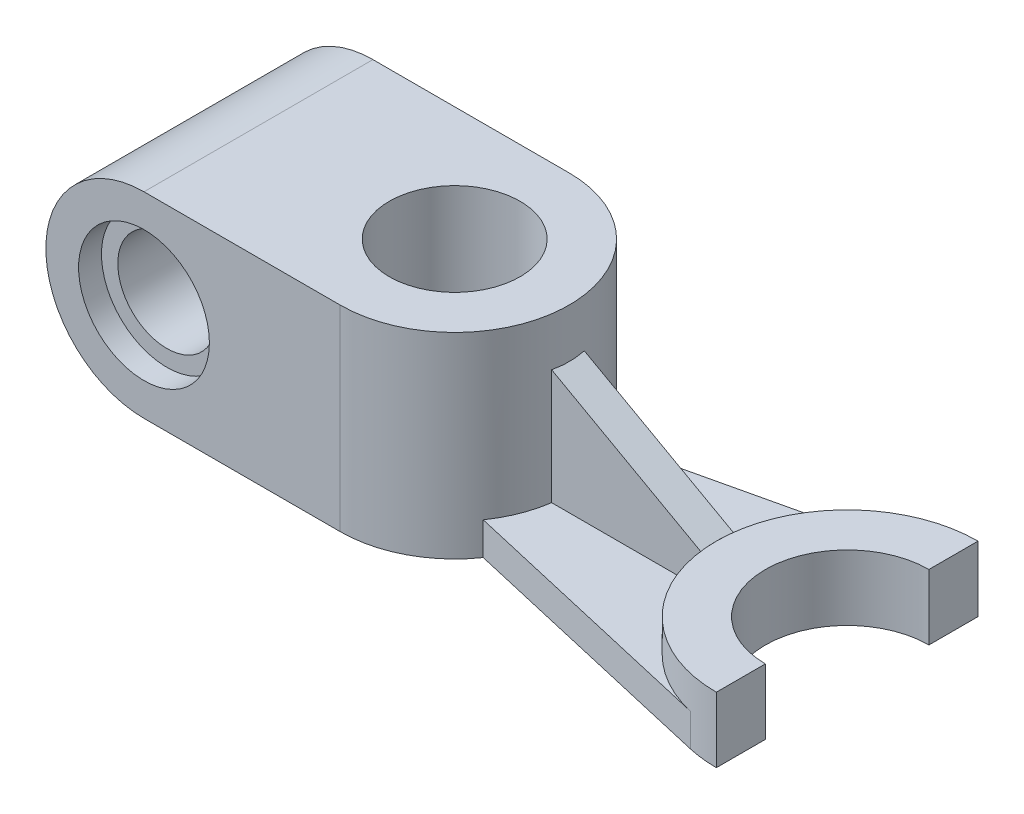
ISO-10303-21;
HEADER;
FILE_DESCRIPTION(('STEP AP214'),'2;1');
FILE_NAME('part.step','',(''),(''),'','','');
FILE_SCHEMA(('AUTOMOTIVE_DESIGN { 1 0 10303 214 1 1 1 1 }'));
ENDSEC;
DATA;
#1=APPLICATION_CONTEXT('core data for automotive mechanical design processes');
#2=APPLICATION_PROTOCOL_DEFINITION('international standard','automotive_design',2000,#1);
#3=PRODUCT_CONTEXT('',#1,'mechanical');
#4=PRODUCT('Part','Part','',(#3));
#5=PRODUCT_RELATED_PRODUCT_CATEGORY('part','',(#4));
#6=PRODUCT_DEFINITION_FORMATION('','',#4);
#7=PRODUCT_DEFINITION_CONTEXT('part definition',#1,'design');
#8=PRODUCT_DEFINITION('design','',#6,#7);
#9=PRODUCT_DEFINITION_SHAPE('','',#8);
#10=(LENGTH_UNIT() NAMED_UNIT(*) SI_UNIT(.MILLI.,.METRE.));
#11=(NAMED_UNIT(*) PLANE_ANGLE_UNIT() SI_UNIT($,.RADIAN.));
#12=(NAMED_UNIT(*) SI_UNIT($,.STERADIAN.) SOLID_ANGLE_UNIT());
#13=UNCERTAINTY_MEASURE_WITH_UNIT(LENGTH_MEASURE(1.E-05),#10,'distance_accuracy_value','');
#14=(GEOMETRIC_REPRESENTATION_CONTEXT(3) GLOBAL_UNCERTAINTY_ASSIGNED_CONTEXT((#13)) GLOBAL_UNIT_ASSIGNED_CONTEXT((#10,
#11,#12)) REPRESENTATION_CONTEXT('',''));
#15=CARTESIAN_POINT('',(0.,0.,0.));
#16=DIRECTION('',(0.,0.,1.));
#17=DIRECTION('',(1.,0.,0.));
#18=AXIS2_PLACEMENT_3D('',#15,#16,#17);
#19=CARTESIAN_POINT('',(0.,10.,0.));
#20=DIRECTION('',(0.,1.,0.));
#21=DIRECTION('',(0.,0.,1.));
#22=AXIS2_PLACEMENT_3D('',#19,#20,#21);
#23=PLANE('',#22);
#24=CARTESIAN_POINT('',(0.,10.,0.));
#25=DIRECTION('',(0.,-1.,0.));
#26=DIRECTION('',(0.,0.,1.));
#27=AXIS2_PLACEMENT_3D('',#24,#25,#26);
#28=CIRCLE('',#27,35.);
#29=CARTESIAN_POINT('',(28.7228132326901,10.,-20.));
#30=VERTEX_POINT('',#29);
#31=CARTESIAN_POINT('',(34.6410161513775,10.,-5.));
#32=VERTEX_POINT('',#31);
#33=EDGE_CURVE('E166',#30,#32,#28,.T.);
#34=ORIENTED_EDGE('',*,*,#33,.T.);
#35=DIRECTION('',(1.,0.,0.));
#36=VECTOR('',#35,1.);
#37=CARTESIAN_POINT('',(0.,10.,-5.));
#38=LINE('',#37,#36);
#39=CARTESIAN_POINT('',(80.3137303340311,10.,-5.));
#40=VERTEX_POINT('',#39);
#41=EDGE_CURVE('E170',#32,#40,#38,.T.);
#42=ORIENTED_EDGE('',*,*,#41,.T.);
#43=CARTESIAN_POINT('',(120.,10.,0.));
#44=DIRECTION('',(0.,-1.,0.));
#45=DIRECTION('',(0.,0.,1.));
#46=AXIS2_PLACEMENT_3D('',#43,#44,#45);
#47=CIRCLE('',#46,40.);
#48=CARTESIAN_POINT('',(111.011327844652,10.,-38.9769646443084));
#49=VERTEX_POINT('',#48);
#50=EDGE_CURVE('E155',#40,#49,#47,.T.);
#51=ORIENTED_EDGE('',*,*,#50,.T.);
#52=DIRECTION('',(-0.97442411610771,0.,0.224716803883704));
#53=VECTOR('',#52,1.);
#54=CARTESIAN_POINT('',(111.011327844652,10.,-38.9769646443084));
#55=LINE('',#54,#53);
#56=EDGE_CURVE('E245',#49,#30,#55,.T.);
#57=ORIENTED_EDGE('',*,*,#56,.T.);
#58=EDGE_LOOP('',(#34,#42,#51,#57));
#59=FACE_BOUND('',#58,.T.);
#60=ADVANCED_FACE('F39',(#59),#23,.T.);
#61=CARTESIAN_POINT('',(120.,20.,0.));
#62=DIRECTION('',(0.,-1.,0.));
#63=DIRECTION('',(0.,0.,-1.));
#64=AXIS2_PLACEMENT_3D('',#61,#62,#63);
#65=CYLINDRICAL_SURFACE('',#64,40.);
#66=CARTESIAN_POINT('',(120.,-2.22222222222223,0.));
#67=DIRECTION('',(-0.485642931178632,-0.874157276121538,0.));
#68=DIRECTION('',(0.874157276121538,-0.485642931178632,0.));
#69=AXIS2_PLACEMENT_3D('',#66,#67,#68);
#70=ELLIPSE('',#69,45.7583561821644,40.);
#71=CARTESIAN_POINT('',(80.,20.,0.));
#72=VERTEX_POINT('',#71);
#73=CARTESIAN_POINT('',(80.3137303340311,19.8257053699827,5.));
#74=VERTEX_POINT('',#73);
#75=EDGE_CURVE('E295',#72,#74,#70,.F.);
#76=ORIENTED_EDGE('',*,*,#75,.T.);
#77=DIRECTION('',(0.,-1.,0.));
#78=VECTOR('',#77,1.);
#79=CARTESIAN_POINT('',(80.3137303340311,20.,5.));
#80=LINE('',#79,#78);
#81=CARTESIAN_POINT('',(80.3137303340311,10.,5.));
#82=VERTEX_POINT('',#81);
#83=EDGE_CURVE('E11',#74,#82,#80,.T.);
#84=ORIENTED_EDGE('',*,*,#83,.T.);
#85=CARTESIAN_POINT('',(111.011327844652,10.,38.9769646443084));
#86=VERTEX_POINT('',#85);
#87=EDGE_CURVE('E162',#86,#82,#47,.T.);
#88=ORIENTED_EDGE('',*,*,#87,.F.);
#89=DIRECTION('',(0.,-1.,0.));
#90=VECTOR('',#89,1.);
#91=CARTESIAN_POINT('',(111.011327844652,10.,38.9769646443084));
#92=LINE('',#91,#90);
#93=CARTESIAN_POINT('',(111.011327844652,0.,38.9769646443084));
#94=VERTEX_POINT('',#93);
#95=EDGE_CURVE('E236',#86,#94,#92,.T.);
#96=ORIENTED_EDGE('',*,*,#95,.T.);
#97=CARTESIAN_POINT('',(120.,0.,0.));
#98=DIRECTION('',(0.,1.,0.));
#99=DIRECTION('',(0.,0.,1.));
#100=AXIS2_PLACEMENT_3D('',#97,#98,#99);
#101=CIRCLE('',#100,40.);
#102=CARTESIAN_POINT('',(120.,0.,40.));
#103=VERTEX_POINT('',#102);
#104=EDGE_CURVE('E271',#94,#103,#101,.T.);
#105=ORIENTED_EDGE('',*,*,#104,.T.);
#106=DIRECTION('',(0.,-1.,0.));
#107=VECTOR('',#106,1.);
#108=CARTESIAN_POINT('',(120.,20.,40.));
#109=LINE('',#108,#107);
#110=CARTESIAN_POINT('',(120.,20.,40.));
#111=VERTEX_POINT('',#110);
#112=EDGE_CURVE('E261',#111,#103,#109,.T.);
#113=ORIENTED_EDGE('',*,*,#112,.F.);
#114=CARTESIAN_POINT('',(120.,20.,0.));
#115=DIRECTION('',(0.,1.,0.));
#116=DIRECTION('',(0.,0.,1.));
#117=AXIS2_PLACEMENT_3D('',#114,#115,#116);
#118=CIRCLE('',#117,40.);
#119=EDGE_CURVE('E285',#72,#111,#118,.T.);
#120=ORIENTED_EDGE('',*,*,#119,.F.);
#121=EDGE_LOOP('',(#76,#84,#88,#96,#105,#113,#120));
#122=FACE_BOUND('',#121,.T.);
#123=ADVANCED_FACE('F310',(#122),#65,.T.);
#124=CARTESIAN_POINT('',(0.,60.,0.));
#125=DIRECTION('',(0.,-1.,0.));
#126=DIRECTION('',(0.,0.,-1.));
#127=AXIS2_PLACEMENT_3D('',#124,#125,#126);
#128=CYLINDRICAL_SURFACE('',#127,35.);
#129=CARTESIAN_POINT('',(34.6410161513775,10.,5.));
#130=VERTEX_POINT('',#129);
#131=CARTESIAN_POINT('',(28.7228132326901,10.,20.));
#132=VERTEX_POINT('',#131);
#133=EDGE_CURVE('E246',#130,#132,#28,.T.);
#134=ORIENTED_EDGE('',*,*,#133,.F.);
#135=DIRECTION('',(0.,-1.,0.));
#136=VECTOR('',#135,1.);
#137=CARTESIAN_POINT('',(34.6410161513775,60.,5.));
#138=LINE('',#137,#136);
#139=CARTESIAN_POINT('',(34.6410161513775,45.1994354714569,5.));
#140=VERTEX_POINT('',#139);
#141=EDGE_CURVE('E53',#130,#140,#138,.F.);
#142=ORIENTED_EDGE('',*,*,#141,.T.);
#143=CARTESIAN_POINT('',(0.,64.4444444444444,0.));
#144=DIRECTION('',(-0.485642931178632,-0.874157276121538,0.));
#145=DIRECTION('',(0.874157276121538,-0.485642931178632,0.));
#146=AXIS2_PLACEMENT_3D('',#143,#144,#145);
#147=ELLIPSE('',#146,40.0385616593939,35.);
#148=CARTESIAN_POINT('',(34.6410161513775,45.1994354714569,-5.));
#149=VERTEX_POINT('',#148);
#150=EDGE_CURVE('E59',#140,#149,#147,.F.);
#151=ORIENTED_EDGE('',*,*,#150,.T.);
#152=DIRECTION('',(0.,-1.,0.));
#153=VECTOR('',#152,1.);
#154=CARTESIAN_POINT('',(34.6410161513775,60.,-5.));
#155=LINE('',#154,#153);
#156=EDGE_CURVE('E167',#32,#149,#155,.F.);
#157=ORIENTED_EDGE('',*,*,#156,.F.);
#158=ORIENTED_EDGE('',*,*,#33,.F.);
#159=DIRECTION('',(0.,-1.,0.));
#160=VECTOR('',#159,1.);
#161=CARTESIAN_POINT('',(28.7228132326901,10.,-20.));
#162=LINE('',#161,#160);
#163=CARTESIAN_POINT('',(28.7228132326901,0.,-20.));
#164=VERTEX_POINT('',#163);
#165=EDGE_CURVE('E237',#30,#164,#162,.T.);
#166=ORIENTED_EDGE('',*,*,#165,.T.);
#167=CARTESIAN_POINT('',(0.,0.,0.));
#168=DIRECTION('',(0.,1.,0.));
#169=DIRECTION('',(0.,0.,1.));
#170=AXIS2_PLACEMENT_3D('',#167,#168,#169);
#171=CIRCLE('',#170,35.);
#172=CARTESIAN_POINT('',(0.,0.,-35.));
#173=VERTEX_POINT('',#172);
#174=EDGE_CURVE('E205',#164,#173,#171,.T.);
#175=ORIENTED_EDGE('',*,*,#174,.T.);
#176=DIRECTION('',(0.,-1.,0.));
#177=VECTOR('',#176,1.);
#178=CARTESIAN_POINT('',(0.,60.,-35.));
#179=LINE('',#178,#177);
#180=CARTESIAN_POINT('',(0.,60.,-35.));
#181=VERTEX_POINT('',#180);
#182=EDGE_CURVE('E176',#181,#173,#179,.T.);
#183=ORIENTED_EDGE('',*,*,#182,.F.);
#184=CARTESIAN_POINT('',(0.,60.,0.));
#185=DIRECTION('',(0.,1.,0.));
#186=DIRECTION('',(0.,0.,1.));
#187=AXIS2_PLACEMENT_3D('',#184,#185,#186);
#188=CIRCLE('',#187,35.);
#189=CARTESIAN_POINT('',(0.,60.,35.));
#190=VERTEX_POINT('',#189);
#191=EDGE_CURVE('E196',#190,#181,#188,.T.);
#192=ORIENTED_EDGE('',*,*,#191,.F.);
#193=DIRECTION('',(0.,-1.,0.));
#194=VECTOR('',#193,1.);
#195=CARTESIAN_POINT('',(0.,60.,35.));
#196=LINE('',#195,#194);
#197=CARTESIAN_POINT('',(0.,0.,35.));
#198=VERTEX_POINT('',#197);
#199=EDGE_CURVE('E178',#190,#198,#196,.T.);
#200=ORIENTED_EDGE('',*,*,#199,.T.);
#201=CARTESIAN_POINT('',(28.7228132326901,0.,20.));
#202=VERTEX_POINT('',#201);
#203=EDGE_CURVE('E199',#198,#202,#171,.T.);
#204=ORIENTED_EDGE('',*,*,#203,.T.);
#205=DIRECTION('',(0.,-1.,0.));
#206=VECTOR('',#205,1.);
#207=CARTESIAN_POINT('',(28.7228132326901,10.,20.));
#208=LINE('',#207,#206);
#209=EDGE_CURVE('E233',#132,#202,#208,.T.);
#210=ORIENTED_EDGE('',*,*,#209,.F.);
#211=EDGE_LOOP('',(#134,#142,#151,#157,#158,#166,#175,#183,#192,#200,#204,#210));
#212=FACE_BOUND('',#211,.T.);
#213=ADVANCED_FACE('F41',(#212),#128,.T.);
#214=CARTESIAN_POINT('',(-60.,30.,-35.));
#215=DIRECTION('',(0.,0.,1.));
#216=DIRECTION('',(1.,0.,0.));
#217=AXIS2_PLACEMENT_3D('',#214,#215,#216);
#218=CYLINDRICAL_SURFACE('',#217,15.);
#219=CARTESIAN_POINT('',(-60.,30.,28.));
#220=DIRECTION('',(0.,0.,1.));
#221=DIRECTION('',(1.,0.,0.));
#222=AXIS2_PLACEMENT_3D('',#219,#220,#221);
#223=CIRCLE('',#222,15.);
#224=CARTESIAN_POINT('',(-45.,30.,28.));
#225=VERTEX_POINT('',#224);
#226=EDGE_CURVE('E187',#225,#225,#223,.F.);
#227=ORIENTED_EDGE('',*,*,#226,.F.);
#228=EDGE_LOOP('',(#227));
#229=FACE_BOUND('',#228,.T.);
#230=CARTESIAN_POINT('',(-60.,30.,-28.));
#231=DIRECTION('',(0.,0.,-1.));
#232=DIRECTION('',(-1.,0.,0.));
#233=AXIS2_PLACEMENT_3D('',#230,#231,#232);
#234=CIRCLE('',#233,15.);
#235=CARTESIAN_POINT('',(-75.,30.,-28.));
#236=VERTEX_POINT('',#235);
#237=EDGE_CURVE('E181',#236,#236,#234,.F.);
#238=ORIENTED_EDGE('',*,*,#237,.F.);
#239=EDGE_LOOP('',(#238));
#240=FACE_BOUND('',#239,.T.);
#241=ADVANCED_FACE('F409',(#229,#240),#218,.F.);
#242=CARTESIAN_POINT('',(0.,60.,-35.));
#243=DIRECTION('',(0.,0.,1.));
#244=DIRECTION('',(1.,0.,0.));
#245=AXIS2_PLACEMENT_3D('',#242,#243,#244);
#246=PLANE('',#245);
#247=CARTESIAN_POINT('',(-60.,30.,-35.));
#248=DIRECTION('',(0.,0.,-1.));
#249=DIRECTION('',(-1.,0.,0.));
#250=AXIS2_PLACEMENT_3D('',#247,#248,#249);
#251=CIRCLE('',#250,20.);
#252=CARTESIAN_POINT('',(-80.,30.,-35.));
#253=VERTEX_POINT('',#252);
#254=EDGE_CURVE('E226',#253,#253,#251,.T.);
#255=ORIENTED_EDGE('',*,*,#254,.F.);
#256=EDGE_LOOP('',(#255));
#257=FACE_BOUND('',#256,.T.);
#258=DIRECTION('',(-1.,0.,0.));
#259=VECTOR('',#258,1.);
#260=CARTESIAN_POINT('',(0.,0.,-35.));
#261=LINE('',#260,#259);
#262=CARTESIAN_POINT('',(-60.,0.,-35.));
#263=VERTEX_POINT('',#262);
#264=EDGE_CURVE('E200',#173,#263,#261,.T.);
#265=ORIENTED_EDGE('',*,*,#264,.T.);
#266=CARTESIAN_POINT('',(-60.,30.,-35.));
#267=DIRECTION('',(0.,0.,-1.));
#268=DIRECTION('',(1.,0.,0.));
#269=AXIS2_PLACEMENT_3D('',#266,#267,#268);
#270=CIRCLE('',#269,30.);
#271=CARTESIAN_POINT('',(-60.,60.,-35.));
#272=VERTEX_POINT('',#271);
#273=EDGE_CURVE('E215',#263,#272,#270,.T.);
#274=ORIENTED_EDGE('',*,*,#273,.T.);
#275=DIRECTION('',(-1.,0.,0.));
#276=VECTOR('',#275,1.);
#277=CARTESIAN_POINT('',(0.,60.,-35.));
#278=LINE('',#277,#276);
#279=EDGE_CURVE('E204',#181,#272,#278,.T.);
#280=ORIENTED_EDGE('',*,*,#279,.F.);
#281=ORIENTED_EDGE('',*,*,#182,.T.);
#282=EDGE_LOOP('',(#265,#274,#280,#281));
#283=FACE_BOUND('',#282,.T.);
#284=ADVANCED_FACE('F348',(#257,#283),#246,.F.);
#285=CARTESIAN_POINT('',(-90.,60.,35.));
#286=DIRECTION('',(0.,0.,-1.));
#287=DIRECTION('',(-1.,0.,0.));
#288=AXIS2_PLACEMENT_3D('',#285,#286,#287);
#289=PLANE('',#288);
#290=CARTESIAN_POINT('',(-60.,30.,35.));
#291=DIRECTION('',(0.,0.,1.));
#292=DIRECTION('',(1.,0.,0.));
#293=AXIS2_PLACEMENT_3D('',#290,#291,#292);
#294=CIRCLE('',#293,20.);
#295=CARTESIAN_POINT('',(-40.,30.,35.));
#296=VERTEX_POINT('',#295);
#297=EDGE_CURVE('E183',#296,#296,#294,.T.);
#298=ORIENTED_EDGE('',*,*,#297,.F.);
#299=EDGE_LOOP('',(#298));
#300=FACE_BOUND('',#299,.T.);
#301=CARTESIAN_POINT('',(-60.,30.,35.));
#302=DIRECTION('',(0.,0.,-1.));
#303=DIRECTION('',(1.,0.,0.));
#304=AXIS2_PLACEMENT_3D('',#301,#302,#303);
#305=CIRCLE('',#304,30.);
#306=CARTESIAN_POINT('',(-60.,0.,35.));
#307=VERTEX_POINT('',#306);
#308=CARTESIAN_POINT('',(-60.,60.,35.));
#309=VERTEX_POINT('',#308);
#310=EDGE_CURVE('E211',#307,#309,#305,.T.);
#311=ORIENTED_EDGE('',*,*,#310,.F.);
#312=DIRECTION('',(1.,0.,0.));
#313=VECTOR('',#312,1.);
#314=CARTESIAN_POINT('',(-90.,0.,35.));
#315=LINE('',#314,#313);
#316=EDGE_CURVE('E191',#307,#198,#315,.T.);
#317=ORIENTED_EDGE('',*,*,#316,.T.);
#318=ORIENTED_EDGE('',*,*,#199,.F.);
#319=DIRECTION('',(1.,0.,0.));
#320=VECTOR('',#319,1.);
#321=CARTESIAN_POINT('',(-90.,60.,35.));
#322=LINE('',#321,#320);
#323=EDGE_CURVE('E194',#309,#190,#322,.T.);
#324=ORIENTED_EDGE('',*,*,#323,.F.);
#325=EDGE_LOOP('',(#311,#317,#318,#324));
#326=FACE_BOUND('',#325,.T.);
#327=ADVANCED_FACE('F358',(#300,#326),#289,.F.);
#328=CARTESIAN_POINT('',(0.,60.,0.));
#329=DIRECTION('',(0.,1.,0.));
#330=DIRECTION('',(0.,0.,1.));
#331=AXIS2_PLACEMENT_3D('',#328,#329,#330);
#332=PLANE('',#331);
#333=CARTESIAN_POINT('',(0.,60.,0.));
#334=DIRECTION('',(0.,1.,0.));
#335=DIRECTION('',(0.,0.,1.));
#336=AXIS2_PLACEMENT_3D('',#333,#334,#335);
#337=CIRCLE('',#336,20.);
#338=CARTESIAN_POINT('',(0.,60.,20.));
#339=VERTEX_POINT('',#338);
#340=EDGE_CURVE('E189',#339,#339,#337,.T.);
#341=ORIENTED_EDGE('',*,*,#340,.F.);
#342=EDGE_LOOP('',(#341));
#343=FACE_BOUND('',#342,.T.);
#344=DIRECTION('',(0.,0.,1.));
#345=VECTOR('',#344,1.);
#346=CARTESIAN_POINT('',(-60.,60.,-35.));
#347=LINE('',#346,#345);
#348=EDGE_CURVE('E212',#272,#309,#347,.T.);
#349=ORIENTED_EDGE('',*,*,#348,.T.);
#350=ORIENTED_EDGE('',*,*,#323,.T.);
#351=ORIENTED_EDGE('',*,*,#191,.T.);
#352=ORIENTED_EDGE('',*,*,#279,.T.);
#353=EDGE_LOOP('',(#349,#350,#351,#352));
#354=FACE_BOUND('',#353,.T.);
#355=ADVANCED_FACE('F353',(#343,#354),#332,.T.);
#356=CARTESIAN_POINT('',(0.,0.,0.));
#357=DIRECTION('',(0.,1.,0.));
#358=DIRECTION('',(0.,0.,1.));
#359=AXIS2_PLACEMENT_3D('',#356,#357,#358);
#360=PLANE('',#359);
#361=CARTESIAN_POINT('',(0.,0.,0.));
#362=DIRECTION('',(0.,1.,0.));
#363=DIRECTION('',(0.,0.,1.));
#364=AXIS2_PLACEMENT_3D('',#361,#362,#363);
#365=CIRCLE('',#364,20.);
#366=CARTESIAN_POINT('',(0.,0.,20.));
#367=VERTEX_POINT('',#366);
#368=EDGE_CURVE('E220',#367,#367,#365,.T.);
#369=ORIENTED_EDGE('',*,*,#368,.T.);
#370=EDGE_LOOP('',(#369));
#371=FACE_BOUND('',#370,.T.);
#372=ORIENTED_EDGE('',*,*,#316,.F.);
#373=DIRECTION('',(0.,0.,1.));
#374=VECTOR('',#373,1.);
#375=CARTESIAN_POINT('',(-60.,0.,-35.));
#376=LINE('',#375,#374);
#377=EDGE_CURVE('E209',#263,#307,#376,.T.);
#378=ORIENTED_EDGE('',*,*,#377,.F.);
#379=ORIENTED_EDGE('',*,*,#264,.F.);
#380=ORIENTED_EDGE('',*,*,#174,.F.);
#381=DIRECTION('',(-0.97442411610771,0.,0.224716803883704));
#382=VECTOR('',#381,1.);
#383=CARTESIAN_POINT('',(111.011327844652,0.,-38.9769646443084));
#384=LINE('',#383,#382);
#385=CARTESIAN_POINT('',(111.011327844652,0.,-38.9769646443084));
#386=VERTEX_POINT('',#385);
#387=EDGE_CURVE('E243',#386,#164,#384,.T.);
#388=ORIENTED_EDGE('',*,*,#387,.F.);
#389=CARTESIAN_POINT('',(120.,0.,-40.));
#390=VERTEX_POINT('',#389);
#391=EDGE_CURVE('E272',#390,#386,#101,.T.);
#392=ORIENTED_EDGE('',*,*,#391,.F.);
#393=DIRECTION('',(0.,0.,-1.));
#394=VECTOR('',#393,1.);
#395=CARTESIAN_POINT('',(120.,0.,-40.));
#396=LINE('',#395,#394);
#397=CARTESIAN_POINT('',(120.,0.,-25.));
#398=VERTEX_POINT('',#397);
#399=EDGE_CURVE('E274',#398,#390,#396,.T.);
#400=ORIENTED_EDGE('',*,*,#399,.F.);
#401=CARTESIAN_POINT('',(120.,0.,0.));
#402=DIRECTION('',(0.,-1.,0.));
#403=DIRECTION('',(0.,0.,1.));
#404=AXIS2_PLACEMENT_3D('',#401,#402,#403);
#405=CIRCLE('',#404,25.);
#406=CARTESIAN_POINT('',(120.,0.,25.));
#407=VERTEX_POINT('',#406);
#408=EDGE_CURVE('E277',#407,#398,#405,.T.);
#409=ORIENTED_EDGE('',*,*,#408,.F.);
#410=DIRECTION('',(0.,0.,-1.));
#411=VECTOR('',#410,1.);
#412=CARTESIAN_POINT('',(120.,0.,25.));
#413=LINE('',#412,#411);
#414=EDGE_CURVE('E266',#103,#407,#413,.T.);
#415=ORIENTED_EDGE('',*,*,#414,.F.);
#416=ORIENTED_EDGE('',*,*,#104,.F.);
#417=DIRECTION('',(0.97442411610771,0.,0.224716803883704));
#418=VECTOR('',#417,1.);
#419=CARTESIAN_POINT('',(111.011327844652,0.,38.9769646443084));
#420=LINE('',#419,#418);
#421=EDGE_CURVE('E250',#202,#94,#420,.T.);
#422=ORIENTED_EDGE('',*,*,#421,.F.);
#423=ORIENTED_EDGE('',*,*,#203,.F.);
#424=EDGE_LOOP('',(#372,#378,#379,#380,#388,#392,#400,#409,#415,#416,#422,#423));
#425=FACE_BOUND('',#424,.T.);
#426=ADVANCED_FACE('F325',(#371,#425),#360,.F.);
#427=CARTESIAN_POINT('',(-60.,30.,-35.));
#428=DIRECTION('',(0.,0.,1.));
#429=DIRECTION('',(1.,0.,0.));
#430=AXIS2_PLACEMENT_3D('',#427,#428,#429);
#431=CYLINDRICAL_SURFACE('',#430,30.);
#432=ORIENTED_EDGE('',*,*,#310,.T.);
#433=ORIENTED_EDGE('',*,*,#348,.F.);
#434=ORIENTED_EDGE('',*,*,#273,.F.);
#435=ORIENTED_EDGE('',*,*,#377,.T.);
#436=EDGE_LOOP('',(#432,#433,#434,#435));
#437=FACE_BOUND('',#436,.T.);
#438=ADVANCED_FACE('F356',(#437),#431,.T.);
#439=CARTESIAN_POINT('',(0.,0.,0.));
#440=DIRECTION('',(0.,1.,0.));
#441=DIRECTION('',(0.,0.,1.));
#442=AXIS2_PLACEMENT_3D('',#439,#440,#441);
#443=CYLINDRICAL_SURFACE('',#442,20.);
#444=ORIENTED_EDGE('',*,*,#368,.F.);
#445=EDGE_LOOP('',(#444));
#446=FACE_BOUND('',#445,.T.);
#447=ORIENTED_EDGE('',*,*,#340,.T.);
#448=EDGE_LOOP('',(#447));
#449=FACE_BOUND('',#448,.T.);
#450=ADVANCED_FACE('F359',(#446,#449),#443,.F.);
#451=CARTESIAN_POINT('',(-60.,30.,28.));
#452=DIRECTION('',(0.,0.,1.));
#453=DIRECTION('',(1.,0.,0.));
#454=AXIS2_PLACEMENT_3D('',#451,#452,#453);
#455=PLANE('',#454);
#456=CARTESIAN_POINT('',(-60.,30.,28.));
#457=DIRECTION('',(0.,0.,1.));
#458=DIRECTION('',(1.,0.,0.));
#459=AXIS2_PLACEMENT_3D('',#456,#457,#458);
#460=CIRCLE('',#459,20.);
#461=CARTESIAN_POINT('',(-40.,30.,28.));
#462=VERTEX_POINT('',#461);
#463=EDGE_CURVE('E186',#462,#462,#460,.T.);
#464=ORIENTED_EDGE('',*,*,#463,.T.);
#465=EDGE_LOOP('',(#464));
#466=FACE_BOUND('',#465,.T.);
#467=ORIENTED_EDGE('',*,*,#226,.T.);
#468=EDGE_LOOP('',(#467));
#469=FACE_BOUND('',#468,.T.);
#470=ADVANCED_FACE('F366',(#466,#469),#455,.T.);
#471=CARTESIAN_POINT('',(-60.,30.,28.));
#472=DIRECTION('',(0.,0.,1.));
#473=DIRECTION('',(1.,0.,0.));
#474=AXIS2_PLACEMENT_3D('',#471,#472,#473);
#475=CYLINDRICAL_SURFACE('',#474,20.);
#476=ORIENTED_EDGE('',*,*,#463,.F.);
#477=EDGE_LOOP('',(#476));
#478=FACE_BOUND('',#477,.T.);
#479=ORIENTED_EDGE('',*,*,#297,.T.);
#480=EDGE_LOOP('',(#479));
#481=FACE_BOUND('',#480,.T.);
#482=ADVANCED_FACE('F400',(#478,#481),#475,.F.);
#483=CARTESIAN_POINT('',(-60.,30.,-28.));
#484=DIRECTION('',(0.,0.,-1.));
#485=DIRECTION('',(-1.,0.,0.));
#486=AXIS2_PLACEMENT_3D('',#483,#484,#485);
#487=PLANE('',#486);
#488=CARTESIAN_POINT('',(-60.,30.,-28.));
#489=DIRECTION('',(0.,0.,-1.));
#490=DIRECTION('',(-1.,0.,0.));
#491=AXIS2_PLACEMENT_3D('',#488,#489,#490);
#492=CIRCLE('',#491,20.);
#493=CARTESIAN_POINT('',(-80.,30.,-28.));
#494=VERTEX_POINT('',#493);
#495=EDGE_CURVE('E184',#494,#494,#492,.T.);
#496=ORIENTED_EDGE('',*,*,#495,.T.);
#497=EDGE_LOOP('',(#496));
#498=FACE_BOUND('',#497,.T.);
#499=ORIENTED_EDGE('',*,*,#237,.T.);
#500=EDGE_LOOP('',(#499));
#501=FACE_BOUND('',#500,.T.);
#502=ADVANCED_FACE('F393',(#498,#501),#487,.T.);
#503=CARTESIAN_POINT('',(-60.,30.,-28.));
#504=DIRECTION('',(0.,0.,-1.));
#505=DIRECTION('',(-1.,0.,0.));
#506=AXIS2_PLACEMENT_3D('',#503,#504,#505);
#507=CYLINDRICAL_SURFACE('',#506,20.);
#508=ORIENTED_EDGE('',*,*,#495,.F.);
#509=EDGE_LOOP('',(#508));
#510=FACE_BOUND('',#509,.T.);
#511=ORIENTED_EDGE('',*,*,#254,.T.);
#512=EDGE_LOOP('',(#511));
#513=FACE_BOUND('',#512,.T.);
#514=ADVANCED_FACE('F391',(#510,#513),#507,.F.);
#515=CARTESIAN_POINT('',(111.011327844652,10.,38.9769646443084));
#516=DIRECTION('',(0.224716803883704,0.,-0.974424116107711));
#517=DIRECTION('',(-0.974424116107711,0.,-0.224716803883704));
#518=AXIS2_PLACEMENT_3D('',#515,#516,#517);
#519=PLANE('',#518);
#520=ORIENTED_EDGE('',*,*,#421,.T.);
#521=ORIENTED_EDGE('',*,*,#95,.F.);
#522=DIRECTION('',(0.97442411610771,0.,0.224716803883704));
#523=VECTOR('',#522,1.);
#524=CARTESIAN_POINT('',(111.011327844652,10.,38.9769646443084));
#525=LINE('',#524,#523);
#526=EDGE_CURVE('E161',#132,#86,#525,.T.);
#527=ORIENTED_EDGE('',*,*,#526,.F.);
#528=ORIENTED_EDGE('',*,*,#209,.T.);
#529=EDGE_LOOP('',(#520,#521,#527,#528));
#530=FACE_BOUND('',#529,.T.);
#531=ADVANCED_FACE('F314',(#530),#519,.F.);
#532=CARTESIAN_POINT('',(111.011327844652,10.,-38.9769646443084));
#533=DIRECTION('',(0.224716803883704,0.,0.974424116107711));
#534=DIRECTION('',(0.974424116107711,0.,-0.224716803883704));
#535=AXIS2_PLACEMENT_3D('',#532,#533,#534);
#536=PLANE('',#535);
#537=ORIENTED_EDGE('',*,*,#387,.T.);
#538=ORIENTED_EDGE('',*,*,#165,.F.);
#539=ORIENTED_EDGE('',*,*,#56,.F.);
#540=DIRECTION('',(0.,-1.,0.));
#541=VECTOR('',#540,1.);
#542=CARTESIAN_POINT('',(111.011327844652,10.,-38.9769646443084));
#543=LINE('',#542,#541);
#544=EDGE_CURVE('E156',#49,#386,#543,.T.);
#545=ORIENTED_EDGE('',*,*,#544,.T.);
#546=EDGE_LOOP('',(#537,#538,#539,#545));
#547=FACE_BOUND('',#546,.T.);
#548=ADVANCED_FACE('F341',(#547),#536,.F.);
#549=DIRECTION('',(1.,0.,0.));
#550=VECTOR('',#549,1.);
#551=CARTESIAN_POINT('',(0.,10.,5.));
#552=LINE('',#551,#550);
#553=EDGE_CURVE('E286',#130,#82,#552,.T.);
#554=ORIENTED_EDGE('',*,*,#553,.F.);
#555=ORIENTED_EDGE('',*,*,#133,.T.);
#556=ORIENTED_EDGE('',*,*,#526,.T.);
#557=ORIENTED_EDGE('',*,*,#87,.T.);
#558=EDGE_LOOP('',(#554,#555,#556,#557));
#559=FACE_BOUND('',#558,.T.);
#560=ADVANCED_FACE('F309',(#559),#23,.T.);
#561=CARTESIAN_POINT('',(120.,20.,0.));
#562=DIRECTION('',(0.,-1.,0.));
#563=DIRECTION('',(0.,0.,-1.));
#564=AXIS2_PLACEMENT_3D('',#561,#562,#563);
#565=CYLINDRICAL_SURFACE('',#564,25.);
#566=ORIENTED_EDGE('',*,*,#408,.T.);
#567=DIRECTION('',(0.,-1.,0.));
#568=VECTOR('',#567,1.);
#569=CARTESIAN_POINT('',(120.,20.,-25.));
#570=LINE('',#569,#568);
#571=CARTESIAN_POINT('',(120.,20.,-25.));
#572=VERTEX_POINT('',#571);
#573=EDGE_CURVE('E249',#572,#398,#570,.T.);
#574=ORIENTED_EDGE('',*,*,#573,.F.);
#575=CARTESIAN_POINT('',(120.,20.,0.));
#576=DIRECTION('',(0.,-1.,0.));
#577=DIRECTION('',(0.,0.,1.));
#578=AXIS2_PLACEMENT_3D('',#575,#576,#577);
#579=CIRCLE('',#578,25.);
#580=CARTESIAN_POINT('',(120.,20.,25.));
#581=VERTEX_POINT('',#580);
#582=EDGE_CURVE('E267',#581,#572,#579,.T.);
#583=ORIENTED_EDGE('',*,*,#582,.F.);
#584=DIRECTION('',(0.,-1.,0.));
#585=VECTOR('',#584,1.);
#586=CARTESIAN_POINT('',(120.,20.,25.));
#587=LINE('',#586,#585);
#588=EDGE_CURVE('E263',#581,#407,#587,.T.);
#589=ORIENTED_EDGE('',*,*,#588,.T.);
#590=EDGE_LOOP('',(#566,#574,#583,#589));
#591=FACE_BOUND('',#590,.T.);
#592=ADVANCED_FACE('F335',(#591),#565,.F.);
#593=CARTESIAN_POINT('',(120.,20.,-40.));
#594=DIRECTION('',(-1.,0.,0.));
#595=DIRECTION('',(0.,0.,1.));
#596=AXIS2_PLACEMENT_3D('',#593,#594,#595);
#597=PLANE('',#596);
#598=ORIENTED_EDGE('',*,*,#399,.T.);
#599=DIRECTION('',(0.,-1.,0.));
#600=VECTOR('',#599,1.);
#601=CARTESIAN_POINT('',(120.,20.,-40.));
#602=LINE('',#601,#600);
#603=CARTESIAN_POINT('',(120.,20.,-40.));
#604=VERTEX_POINT('',#603);
#605=EDGE_CURVE('E259',#604,#390,#602,.T.);
#606=ORIENTED_EDGE('',*,*,#605,.F.);
#607=DIRECTION('',(0.,0.,-1.));
#608=VECTOR('',#607,1.);
#609=CARTESIAN_POINT('',(120.,20.,-40.));
#610=LINE('',#609,#608);
#611=EDGE_CURVE('E282',#572,#604,#610,.T.);
#612=ORIENTED_EDGE('',*,*,#611,.F.);
#613=ORIENTED_EDGE('',*,*,#573,.T.);
#614=EDGE_LOOP('',(#598,#606,#612,#613));
#615=FACE_BOUND('',#614,.T.);
#616=ADVANCED_FACE('F383',(#615),#597,.F.);
#617=DIRECTION('',(0.,-1.,0.));
#618=VECTOR('',#617,1.);
#619=CARTESIAN_POINT('',(80.3137303340311,20.,-5.));
#620=LINE('',#619,#618);
#621=CARTESIAN_POINT('',(80.3137303340311,19.8257053699827,-5.));
#622=VERTEX_POINT('',#621);
#623=EDGE_CURVE('E50',#622,#40,#620,.T.);
#624=ORIENTED_EDGE('',*,*,#623,.F.);
#625=EDGE_CURVE('E291',#622,#72,#70,.F.);
#626=ORIENTED_EDGE('',*,*,#625,.T.);
#627=EDGE_CURVE('E276',#604,#72,#118,.T.);
#628=ORIENTED_EDGE('',*,*,#627,.F.);
#629=ORIENTED_EDGE('',*,*,#605,.T.);
#630=ORIENTED_EDGE('',*,*,#391,.T.);
#631=ORIENTED_EDGE('',*,*,#544,.F.);
#632=ORIENTED_EDGE('',*,*,#50,.F.);
#633=EDGE_LOOP('',(#624,#626,#628,#629,#630,#631,#632));
#634=FACE_BOUND('',#633,.T.);
#635=ADVANCED_FACE('F153',(#634),#65,.T.);
#636=CARTESIAN_POINT('',(120.,20.,25.));
#637=DIRECTION('',(-1.,0.,0.));
#638=DIRECTION('',(0.,0.,1.));
#639=AXIS2_PLACEMENT_3D('',#636,#637,#638);
#640=PLANE('',#639);
#641=ORIENTED_EDGE('',*,*,#414,.T.);
#642=ORIENTED_EDGE('',*,*,#588,.F.);
#643=DIRECTION('',(0.,0.,-1.));
#644=VECTOR('',#643,1.);
#645=CARTESIAN_POINT('',(120.,20.,25.));
#646=LINE('',#645,#644);
#647=EDGE_CURVE('E270',#111,#581,#646,.T.);
#648=ORIENTED_EDGE('',*,*,#647,.F.);
#649=ORIENTED_EDGE('',*,*,#112,.T.);
#650=EDGE_LOOP('',(#641,#642,#648,#649));
#651=FACE_BOUND('',#650,.T.);
#652=ADVANCED_FACE('F327',(#651),#640,.F.);
#653=CARTESIAN_POINT('',(120.,20.,0.));
#654=DIRECTION('',(0.,1.,0.));
#655=DIRECTION('',(0.,0.,1.));
#656=AXIS2_PLACEMENT_3D('',#653,#654,#655);
#657=PLANE('',#656);
#658=ORIENTED_EDGE('',*,*,#582,.T.);
#659=ORIENTED_EDGE('',*,*,#611,.T.);
#660=ORIENTED_EDGE('',*,*,#627,.T.);
#661=ORIENTED_EDGE('',*,*,#119,.T.);
#662=ORIENTED_EDGE('',*,*,#647,.T.);
#663=EDGE_LOOP('',(#658,#659,#660,#661,#662));
#664=FACE_BOUND('',#663,.T.);
#665=ADVANCED_FACE('F332',(#664),#657,.T.);
#666=CARTESIAN_POINT('',(15.,30.,5.));
#667=DIRECTION('',(0.,0.,1.));
#668=DIRECTION('',(1.,0.,0.));
#669=AXIS2_PLACEMENT_3D('',#666,#667,#668);
#670=PLANE('',#669);
#671=ORIENTED_EDGE('',*,*,#141,.F.);
#672=ORIENTED_EDGE('',*,*,#553,.T.);
#673=ORIENTED_EDGE('',*,*,#83,.F.);
#674=DIRECTION('',(0.874157276121538,-0.485642931178632,0.));
#675=VECTOR('',#674,1.);
#676=CARTESIAN_POINT('',(35.,45.,5.));
#677=LINE('',#676,#675);
#678=EDGE_CURVE('E298',#140,#74,#677,.T.);
#679=ORIENTED_EDGE('',*,*,#678,.F.);
#680=EDGE_LOOP('',(#671,#672,#673,#679));
#681=FACE_BOUND('',#680,.T.);
#682=ADVANCED_FACE('F304',(#681),#670,.T.);
#683=CARTESIAN_POINT('',(15.,30.,-5.));
#684=DIRECTION('',(0.,0.,1.));
#685=DIRECTION('',(1.,0.,0.));
#686=AXIS2_PLACEMENT_3D('',#683,#684,#685);
#687=PLANE('',#686);
#688=ORIENTED_EDGE('',*,*,#41,.F.);
#689=ORIENTED_EDGE('',*,*,#156,.T.);
#690=DIRECTION('',(0.874157276121538,-0.485642931178632,0.));
#691=VECTOR('',#690,1.);
#692=CARTESIAN_POINT('',(35.,45.,-5.));
#693=LINE('',#692,#691);
#694=EDGE_CURVE('E174',#149,#622,#693,.T.);
#695=ORIENTED_EDGE('',*,*,#694,.T.);
#696=ORIENTED_EDGE('',*,*,#623,.T.);
#697=EDGE_LOOP('',(#688,#689,#695,#696));
#698=FACE_BOUND('',#697,.T.);
#699=ADVANCED_FACE('F173',(#698),#687,.F.);
#700=CARTESIAN_POINT('',(35.,45.,0.));
#701=DIRECTION('',(-0.485642931178632,-0.874157276121538,0.));
#702=DIRECTION('',(0.874157276121538,-0.485642931178632,0.));
#703=AXIS2_PLACEMENT_3D('',#700,#701,#702);
#704=PLANE('',#703);
#705=ORIENTED_EDGE('',*,*,#150,.F.);
#706=ORIENTED_EDGE('',*,*,#678,.T.);
#707=ORIENTED_EDGE('',*,*,#75,.F.);
#708=ORIENTED_EDGE('',*,*,#625,.F.);
#709=ORIENTED_EDGE('',*,*,#694,.F.);
#710=EDGE_LOOP('',(#705,#706,#707,#708,#709));
#711=FACE_BOUND('',#710,.T.);
#712=ADVANCED_FACE('F305',(#711),#704,.F.);
#713=CLOSED_SHELL('',(#60,#123,#213,#241,#284,#327,#355,#426,#438,#450,#470,#482,#502,#514,#531,
#548,#560,#592,#616,#635,#652,#665,#682,#699,#712));
#714=MANIFOLD_SOLID_BREP('B2',#713);
#715=ADVANCED_BREP_SHAPE_REPRESENTATION('',(#18,#714),#14);
#716=SHAPE_DEFINITION_REPRESENTATION(#9,#715);
ENDSEC;
END-ISO-10303-21;
